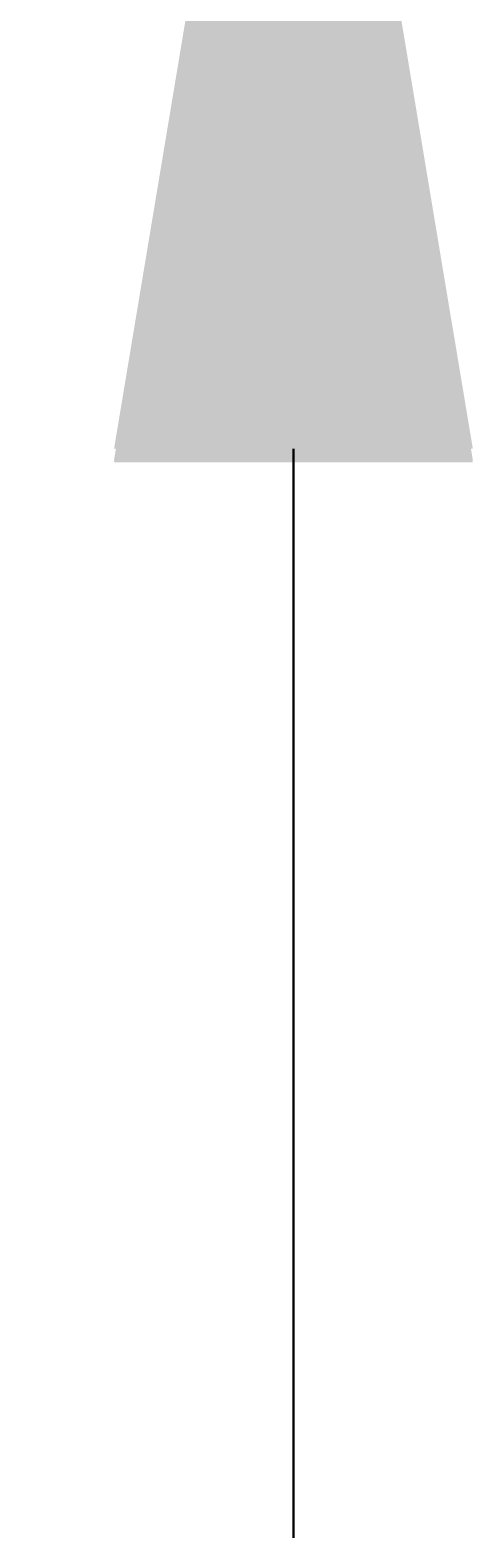
# Model space of a CAD drawing. Units: millimetres. Extents: x -22994 to 29398, y -19990 to 20176.
# Tile 2 of 135: x -2139 to 1973, y -19990 to -5973. Entities that reach past the tile are written whole.
import ezdxf

# ---------------------------------------------------------------- set-up
doc = ezdxf.new("R2010")
doc.units = ezdxf.units.MM
doc.header["$MEASUREMENT"] = 0
doc.layers.add('M-DIMS', color=2, linetype='Continuous', lineweight=18)
doc.styles.get("Standard").update_dxf_attribs({"font": 'arial.ttf'})
doc.dimstyles.get("Standard").update_dxf_attribs({"dimtxt": 0.18, "dimasz": 10000, "dimexe": 0.18, "dimexo": 0.0625, "dimgap": 0.09, "dimtad": 0, "dimtih": 1, "dimtoh": 1, "dimdec": 0, "dimzin": 0, "dimdsep": 46, "dimtxsty": 'Standard', "dimcen": 0.09, "dimadec": 0, "dimazin": 0, "dimtfac": 1, "dimtdec": 0, "dimtofl": 0, "dimtmove": 0, "dimatfit": 3, "dimfxl": 1, "dimtolj": 1, "dimtzin": 0, "dimlwd": 30, "dimarcsym": 0})

# ---------------------------------------------------------------- blocks, each defined once
blk = doc.blocks.new('*D9')
at = {"layer": 'Defpoints', "color": 0, "transparency": 16777216}
for p in [(187, 176), (306, 176), (291, 10)]:
    blk.add_point(p, dxfattribs=at)
at = {"layer": 'M-DIMS', "color": 0, "lineweight": 30, "transparency": 16777216}
for p, q in [((306, 10176), (306, 20176)), ((306, -9990), (306, -19990))]:
    blk.add_line(p, q, dxfattribs=at)
at = {"layer": 'M-DIMS', "color": 0, "lineweight": -2, "transparency": 16777216}
for p, q in [((187, 176), (306, 176)), ((291, 10), (306, 10))]:
    blk.add_line(p, q, dxfattribs=at)
at = {"layer": 'M-DIMS', "color": 0, "transparency": 16777216}
for points in [[(-1360, 10176), (1973, 10176), (306, 176)], [(-1360, -9990), (1973, -9990), (306, 10)]]:
    blk.add_solid(points, dxfattribs=at)
at = {"layer": 'M-DIMS', "color": 0, "transparency": 16777216, "insert": (306, 93), "char_height": 0.18, "attachment_point": 5}
blk.add_mtext('\\A1;166.1', dxfattribs=at)
blk = doc.blocks.new('*D15')
at = {"layer": 'Defpoints', "color": 0, "transparency": 16777216}
for p in [(173, 155), (173, 136), (306, 136)]:
    blk.add_point(p, dxfattribs=at)
at = {"layer": 'M-DIMS', "color": 0, "lineweight": 30, "transparency": 16777216}
for p, q in [((306, 10155), (306, 20155)), ((306, -9864), (306, -19864))]:
    blk.add_line(p, q, dxfattribs=at)
at = {"layer": 'M-DIMS', "color": 0, "lineweight": -2, "transparency": 16777216}
for p, q in [((173, 155), (306, 155)), ((173, 136), (306, 136))]:
    blk.add_line(p, q, dxfattribs=at)
at = {"layer": 'M-DIMS', "color": 0, "transparency": 16777216}
for points in [[(-1360, 10155), (1973, 10155), (306, 155)], [(-1360, -9864), (1973, -9864), (306, 136)]]:
    blk.add_solid(points, dxfattribs=at)
at = {"layer": 'M-DIMS', "color": 0, "transparency": 16777216, "insert": (306, 145), "char_height": 0.18, "attachment_point": 5}
blk.add_mtext('\\A1;18.717', dxfattribs=at)
blk = doc.blocks.new('*D28')
at = {"layer": 'Defpoints', "color": 0, "transparency": 16777216}
for p in [(188, 48), (188, 31), (306, 48)]:
    blk.add_point(p, dxfattribs=at)
at = {"layer": 'M-DIMS', "color": 0, "lineweight": 30, "transparency": 16777216}
for p, q in [((306, 10048), (306, 20048)), ((306, -9969), (306, -19969))]:
    blk.add_line(p, q, dxfattribs=at)
at = {"layer": 'M-DIMS', "color": 0, "lineweight": -2, "transparency": 16777216}
for p, q in [((188, 48), (306, 48)), ((188, 31), (306, 31))]:
    blk.add_line(p, q, dxfattribs=at)
at = {"layer": 'M-DIMS', "color": 0, "transparency": 16777216}
for points in [[(-1360, 10048), (1973, 10048), (306, 48)], [(-1360, -9969), (1973, -9969), (306, 31)]]:
    blk.add_solid(points, dxfattribs=at)
at = {"layer": 'M-DIMS', "color": 0, "transparency": 16777216, "insert": (306, 40), "char_height": 0.18, "attachment_point": 5}
blk.add_mtext('\\A1;17.045', dxfattribs=at)
blk = doc.blocks.new('*D32')
at = {"layer": 'Defpoints', "color": 0, "transparency": 16777216}
for p in [(52, 113), (57, 119)]:
    blk.add_point(p, dxfattribs=at)
at = {"layer": 'M-DIMS', "color": 0, "lineweight": -2, "transparency": 16777216}
blk.add_line((57, 119), (57, 119), dxfattribs=at)
blk.add_line((57, 119), (57, 119), dxfattribs=at)
at = {"layer": 'M-DIMS', "color": 0, "lineweight": 30, "transparency": 16777216}
for p, q in [((-12993, -15047), (-6470, -7467)), ((-22993, -15047), (-12993, -15047))]:
    blk.add_line(p, q, dxfattribs=at)
at = {"layer": 'M-DIMS', "color": 0, "transparency": 16777216}
blk.add_solid([(-7733, -6380), (-5207, -8554), (52, 113)], dxfattribs=at)
at = {"layer": 'M-DIMS', "color": 0, "transparency": 16777216, "insert": (-22993, -15047), "char_height": 0.18, "attachment_point": 5}
blk.add_mtext('\\A1;2X R7.284', dxfattribs=at)

msp = doc.modelspace()

# ---------------------------------------------------------------- dimensions: what is measured, and where the dimension line sits
at = {"layer": 'M-DIMS'}
for base, p1, p2, override, picture, middle in [((306.202, 176.3662), (290.852, 10.2713), (187.2647, 176.3662), {"dimdec": 1, "dimlfac": 1, "dimrnd": 0, "dimzin": 0, "dimdsep": 46, "dimlunit": 2}, '*D9', (306.202, 93.3187)), ((306.202, 136.0713), (173.3459, 154.788), (173.3459, 136.0713), {"dimdec": 3, "dimlfac": 1, "dimrnd": 0, "dimzin": 0, "dimdsep": 46, "dimlunit": 2}, '*D15', (306.202, 145.4297)), ((306.202, 48.0349), (188.1175, 30.9895), (188.1175, 48.0349), {"dimdec": 3, "dimlfac": 1, "dimrnd": 0, "dimzin": 0, "dimdsep": 46, "dimlunit": 2}, '*D28', (306.202, 39.5122))]:
    dim = msp.add_linear_dim(base=base, p1=p1, p2=p2, angle=90, dimstyle='Standard', override=override, dxfattribs=at)
    dim.commit()
    dim.dimension.update_dxf_attribs({"geometry": picture, "text_midpoint": middle})
dim = msp.add_radius_dim(center=(57.1639, 118.6143), mpoint=(52.4129, 113.0929), text='2X <>', dimstyle='Standard', override={"dimdec": 3, "dimlfac": 1, "dimrnd": 0, "dimzin": 0, "dimdsep": 46, "dimlunit": 2}, dxfattribs=at)
dim.commit()
dim.dimension.update_dxf_attribs({"geometry": '*D32', "text_midpoint": (-22993.208, -15047.0314)})

doc.saveas('drawing.dxf')
